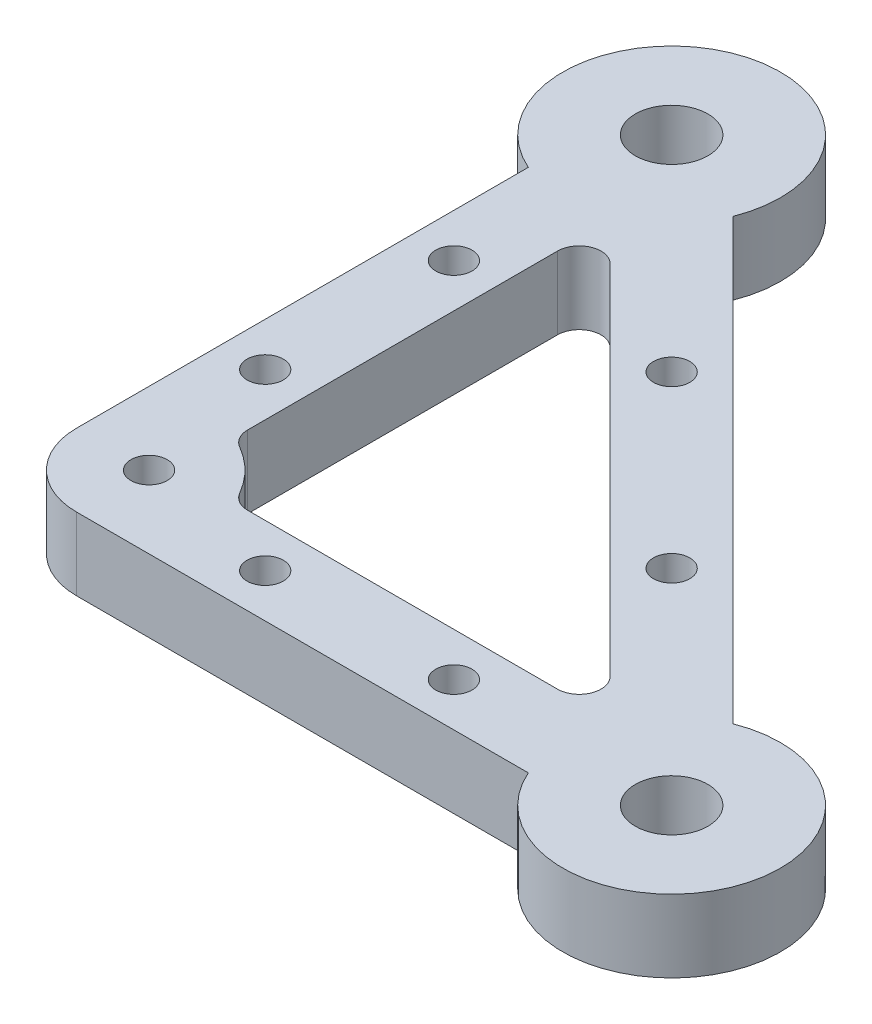
SolidWorks part; units mm, degrees
material "Plain Carbon Steel"
ref_plane "Front Plane" through (0, 0, 0) normal (0, 0, 1) x (1, 0, 0)
ref_plane "Top Plane" through (0, 0, 0) normal (0, 1, 0) x (1, 0, 0)
ref_plane "Right Plane" through (0, 0, 0) normal (1, 0, 0) x (0, 0, -1)
sketch "Web Plate Profile" plane through (0, 0, 0) normal (0, 1, 0) x (1, 0, 0)
  line L0 (0, 0) -> (80, 0) construction
  line L1 (0, 0) -> (0, 80) construction
  line L2 (-6, 4) -> (-6, 66.2523)
  line L3 (4, -6) -> (66.2523, -6)
  line L4 (0, 80) -> (80, 0) construction
  line L5 (13.9638, 74.5215) -> (74.5215, 13.9638)
  line L6 (11.1213, 60.3934) -> (60.3934, 11.1213)
  line L7 (15.5885, 6) -> (58.2721, 6)
  line L8 (6, 15.5885) -> (6, 58.2721)
  arc A0 (-6, 4) -> (4, -6) centre (4, 4) ccw
  arc A1 (66.2523, -6) -> (74.5215, 13.9638) centre (80, 0) ccw
  arc A2 (13.9638, 74.5215) -> (-6, 66.2523) centre (0, 80) ccw
  arc A3 (58.2721, 6) -> (60.3934, 11.1213) centre (58.2721, 9) ccw
  arc A4 (11.1213, 60.3934) -> (6, 58.2721) centre (9, 58.2721) ccw
  arc A5 (15.5885, 6) -> (12.9904, 7.5) centre (15.5885, 9) cw
  arc A6 (12.9904, 7.5) -> (7.5, 12.9904) centre (0, 0) ccw
  arc A7 (7.5, 12.9904) -> (6, 15.5885) centre (9, 15.5885) cw
  circle A8 centre (0, 80) radius 5
  circle A9 centre (80, 0) radius 5
  circle A10 centre (4, 4) radius 2.5
  circle A11 centre (50, 0) radius 2.5
  circle A12 centre (24, 0) radius 2.5
  circle A13 centre (0, 24) radius 2.5
  circle A14 centre (0, 50) radius 2.5
  circle A15 centre (28.2843, 51.7157) radius 2.5
  circle A16 centre (51.7157, 28.2843) radius 2.5
  dimension "D1" = 20
  dimension "D2" = 30
  dimension "D7" = 3
  dimension "D8" = 15
  dimension "D9" = 3
  dimension "D14" = 10
  dimension "D15" = 10
  dimension "D16" = 5
  dimension "D17" = 5
  dimension "D3" = 4
  dimension "D4" = 4
  dimension "D5" = 12
  dimension "D6" = 12
  dimension "D10" = 76
  dimension "D11" = 76
  dimension "D12" = 6
  dimension "D13" = 12
  dimension "D18" = 30
  dimension "D19" = 26
  dimension "D20" = 20
  dimension "D21" = 26
  dimension "D22" = 40
  dimension "D23" = 40
extrude "Web Plate Extrude 10mm" add sketch "Web Plate Profile" along normal mid plane 10
